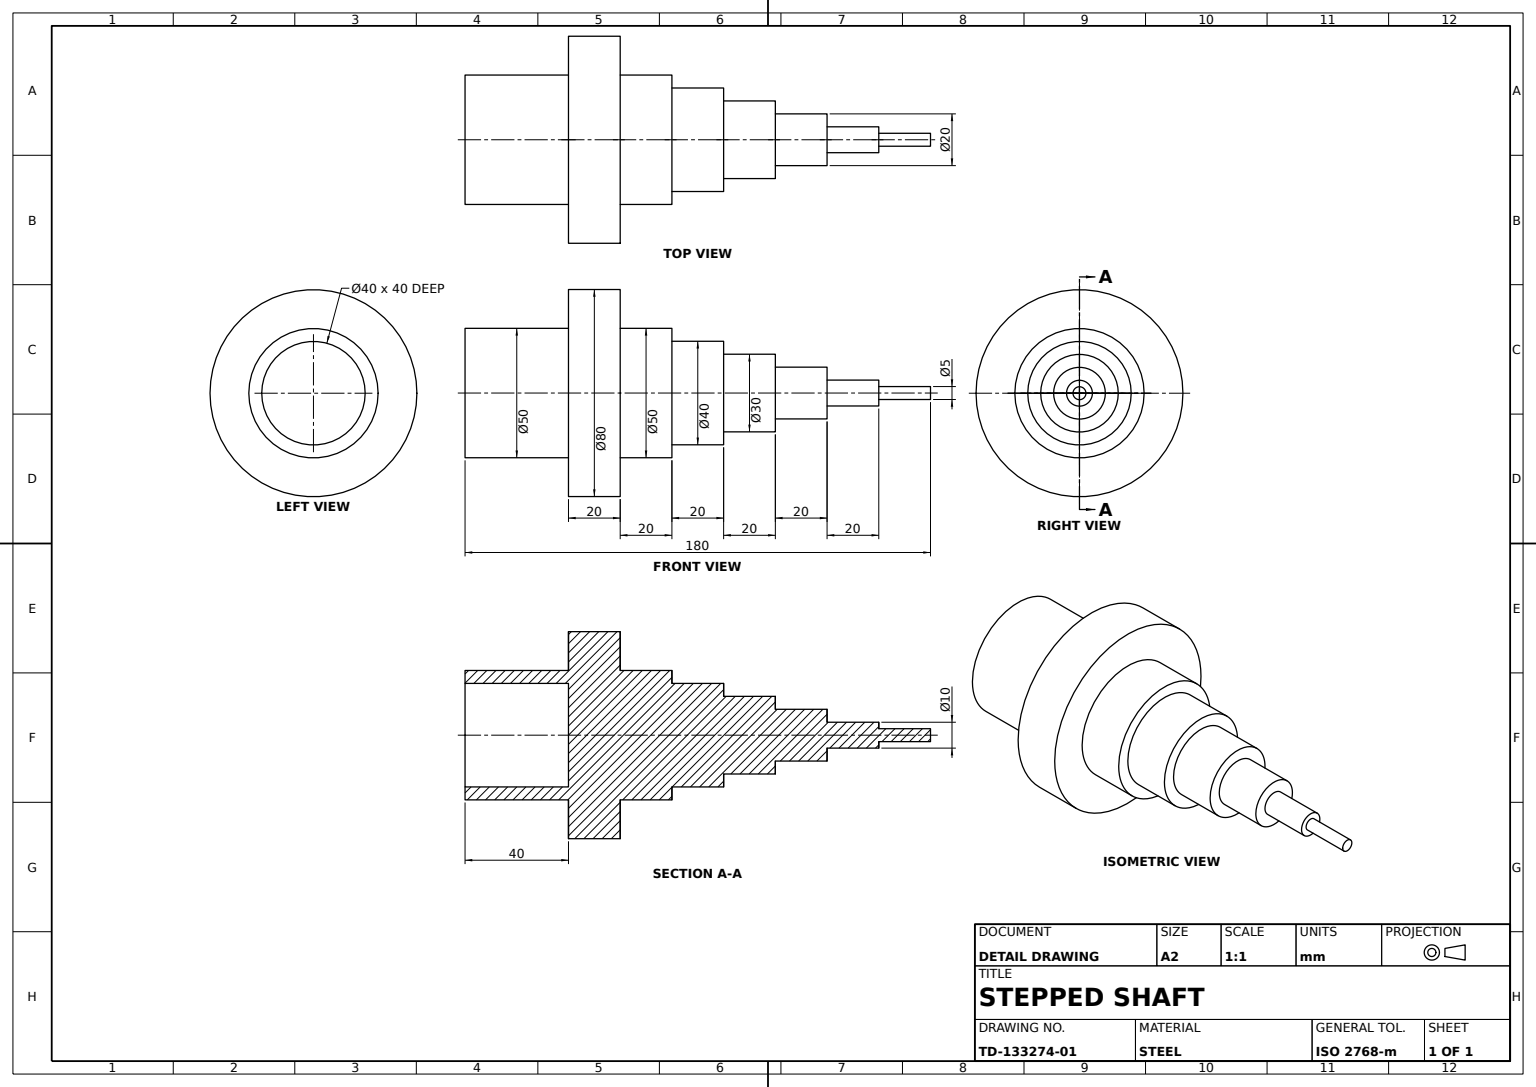
from build123d import *

# Parameters (mm, degrees)
END_START             = -40
END_CUT_SKETCH_40_R   = 20
END_CUT_40_X_40_DEPTH = 40


with BuildPart() as part:
    # Shaft Profile Sketch → Stepped Shaft Revolve (revolve)
    with BuildSketch(Plane.XY, mode=Mode.PRIVATE) as stepped_shaft_revolve_sk:
        Polygon((-40, 0), (-40, 25), (0, 25), (0, 40), (20, 40), (20, 25), (40, 25), (40, 20), (60, 20), (60, 15), (80, 15), (80, 10), (100, 10), (100, 5), (120, 5), (120, 2.5), (140, 2.5), (140, 0), align=None)
    revolve(stepped_shaft_revolve_sk.sketch.rotate(Axis((-63.850651288, 0, 0), (1, 0, 0)), 90), axis=Axis((-63.850651288, 0, 0), (1, 0, 0)))

    # End Cut Sketch Ø40 → End Cut Ø40 x 40 (cut)
    with BuildSketch(Plane.ZY.offset(40).offset(END_START)):
        Circle(END_CUT_SKETCH_40_R)
    extrude(amount=END_CUT_40_X_40_DEPTH, mode=Mode.SUBTRACT)


solid = part.part
